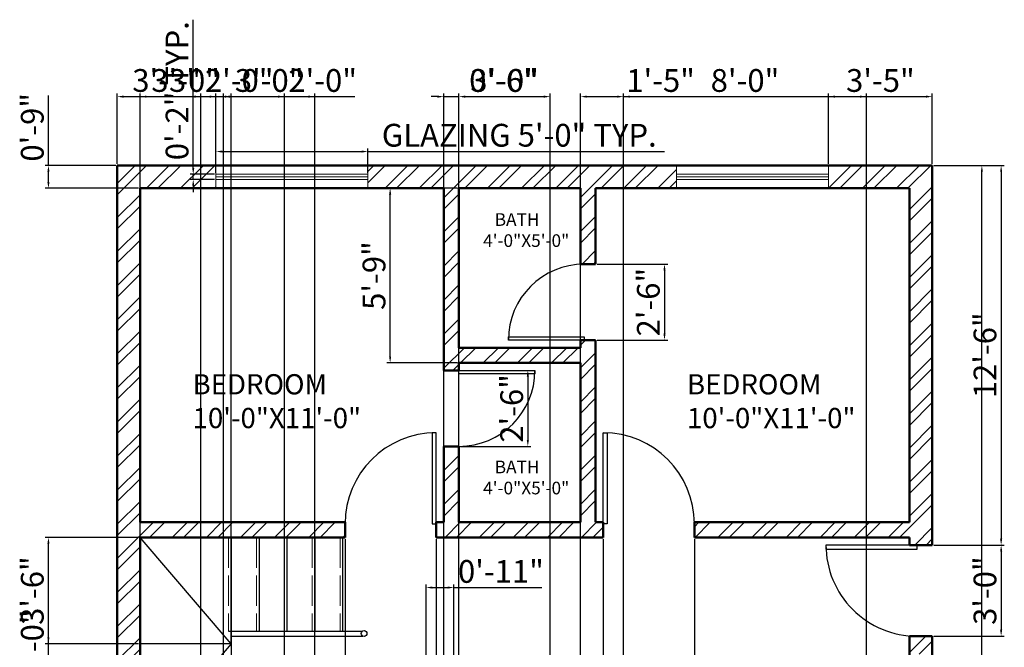
# Model space of a CAD drawing. Units: inches. Extents: x 234 to 630, y 1038 to 1631.
# Tile 2 of 2: x 234 to 623, y 1383 to 1631. Entities that reach past the tile are written whole.
import ezdxf

# ---------------------------------------------------------------- set-up
doc = ezdxf.new("R2010")
doc.units = ezdxf.units.IN
doc.linetypes.add('ACAD_ISO02W100', pattern=[15, 12, -3])
for name, color, linetype, lineweight in [('A-ANNO-DIMS', 2, 'Continuous', 18), ('A-AREA-IDEN', 7, 'Continuous', 25), ('A-DOOR', 4, 'Continuous', 25), ('A-FLOR-STRS', 7, 'Continuous', 25), ('A-FLOR-STRS-HIDN', 8, 'ACAD_ISO02W100', 13), ('A-GLAZ', 244, 'Continuous', 18), ('A-WALL', 7, 'Continuous', 50), ('A-WALL-PATT', 252, 'Continuous', 13)]:
    doc.layers.add(name, color=color, linetype=linetype, lineweight=lineweight)
doc.styles.get("Standard").update_dxf_attribs({"font": 'arial.ttf'})
doc.dimstyles.new('ISO-25', dxfattribs={"dimtxt": 9, "dimasz": 2.5, "dimexe": 1.25, "dimexo": 0.625, "dimtad": 1, "dimlunit": 3, "dimtxsty": 'Standard', "dimcen": 2.5, "dimadec": 0, "dimazin": 0, "dimtfac": 1, "dimtmove": 0, "dimatfit": 3, "dimfxl": 1, "dimarcsym": 0})

# ---------------------------------------------------------------- blocks, each defined once
blk = doc.blocks.new('*U2')
for p, q in [((0, 0), (0, -6)), ((40, 0), (40, -6))]:
    blk.add_line(p, q)
blk.add_lwpolyline([(0, 0), (0, 40), (1.75, 40), (1.75, 0)], close=True)
blk.add_arc((0, 0), 40, 0, 90)
blk = doc.blocks.new('*U4')
for p, q in [((0, 0), (0, -6)), ((-40, 0), (-40, -6))]:
    blk.add_line(p, q)
blk.add_lwpolyline([(0, 0), (0, 40), (-1.75, 40), (-1.75, 0)], close=True)
blk.add_arc((0, 0), 40, 90, 180)
blk = doc.blocks.new('*U5')
for p, q in [((-40, 0), (-40, 6)), ((0, 0), (0, 6))]:
    blk.add_line(p, q)
blk.add_lwpolyline([(0, 0), (0, -40), (-1.75, -40), (-1.75, 0)], close=True)
blk.add_arc((0, 0), 40, 180, 270)
blk = doc.blocks.new('*U3')
for p, q in [((0, 0), (0, 6)), ((40, 0), (40, 6))]:
    blk.add_line(p, q)
blk.add_lwpolyline([(0, 0), (0, -40), (1.75, -40), (1.75, 0)], close=True)
blk.add_arc((0, 0), 40, 270, 0)
blk = doc.blocks.new('*D9')
at = {"layer": 'A-ANNO-DIMS', "color": 0, "lineweight": -2, "transparency": 16777216}
for p, q in [((595.56, 1573.18), (615.76, 1573.18)), ((614.51, 1074.68), (614.51, 1570.68)), ((595.56, 1072.18), (615.76, 1072.18))]:
    blk.add_line(p, q, dxfattribs=at)
at = {"layer": 'A-ANNO-DIMS', "color": 0, "transparency": 16777216}
for points in [[(614.09, 1570.68), (614.92, 1570.68), (614.51, 1573.18)], [(614.09, 1074.68), (614.92, 1074.68), (614.51, 1072.18)]]:
    blk.add_solid(points, dxfattribs=at)
at = {"layer": 'Defpoints', "color": 0, "transparency": 16777216}
for p in [(594.93, 1573.18), (614.51, 1573.18), (594.93, 1072.18)]:
    blk.add_point(p, dxfattribs=at)
at = {"layer": 'A-ANNO-DIMS', "color": 0, "transparency": 16777216, "insert": (609.29, 1322.68), "char_height": 9, "attachment_point": 5, "rotation": 90}
blk.add_mtext('41\'-9"', dxfattribs=at)
blk = doc.blocks.new('WIN-GLAZING-60IN')
for p, q in [((0, 2), (60, 2)), ((0, 1), (60, 1)), ((0, 0), (60, 0))]:
    blk.add_line(p, q)
blk = doc.blocks.new('*D11')
at = {"layer": 'A-ANNO-DIMS', "color": 0, "lineweight": -2, "transparency": 16777216}
for p, q in [((311.93, 1570.3), (311.93, 1579.93)), ((371.93, 1570.3), (371.93, 1579.93)), ((314.43, 1578.68), (369.43, 1578.68)), ((371.93, 1578.68), (489.08, 1578.68))]:
    blk.add_line(p, q, dxfattribs=at)
at = {"layer": 'A-ANNO-DIMS', "color": 0, "transparency": 16777216}
for points in [[(314.43, 1579.1), (314.43, 1578.26), (311.93, 1578.68)], [(369.43, 1579.1), (369.43, 1578.26), (371.93, 1578.68)]]:
    blk.add_solid(points, dxfattribs=at)
at = {"layer": 'Defpoints', "color": 0, "transparency": 16777216}
for p in [(371.93, 1578.68), (311.93, 1569.68), (371.93, 1569.68)]:
    blk.add_point(p, dxfattribs=at)
at = {"layer": 'A-ANNO-DIMS', "color": 0, "transparency": 16777216, "insert": (431.75, 1583.96), "char_height": 9, "attachment_point": 5}
blk.add_mtext('GLAZING 5\'-0" TYP.', dxfattribs=at)
blk = doc.blocks.new('*D12')
at = {"layer": 'A-ANNO-DIMS', "color": 0, "lineweight": -2, "transparency": 16777216}
for p, q in [((302.93, 1572.18), (302.93, 1630.79)), ((311.31, 1569.68), (301.68, 1569.68)), ((302.93, 1567.68), (302.93, 1569.68)), ((311.31, 1567.68), (301.68, 1567.68)), ((302.93, 1565.18), (302.93, 1562.68))]:
    blk.add_line(p, q, dxfattribs=at)
at = {"layer": 'A-ANNO-DIMS', "color": 0, "transparency": 16777216}
for points in [[(302.51, 1572.18), (303.35, 1572.18), (302.93, 1569.68)], [(302.51, 1565.18), (303.35, 1565.18), (302.93, 1567.68)]]:
    blk.add_solid(points, dxfattribs=at)
at = {"layer": 'Defpoints', "color": 0, "transparency": 16777216}
for p in [(302.93, 1569.68), (311.93, 1569.68), (311.93, 1567.68)]:
    blk.add_point(p, dxfattribs=at)
at = {"layer": 'A-ANNO-DIMS', "color": 0, "transparency": 16777216, "insert": (297.71, 1602.73), "char_height": 9, "attachment_point": 5, "rotation": 90}
blk.add_mtext('0\'-2" TYP.', dxfattribs=at)
blk = doc.blocks.new('*D13')
at = {"layer": 'A-ANNO-DIMS', "color": 0, "lineweight": -2, "transparency": 16777216}
for p, q in [((272.93, 1573.8), (272.93, 1601.63)), ((275.43, 1600.38), (309.43, 1600.38)), ((311.93, 1573.8), (311.93, 1601.63))]:
    blk.add_line(p, q, dxfattribs=at)
at = {"layer": 'A-ANNO-DIMS', "color": 0, "transparency": 16777216}
for points in [[(275.43, 1600.8), (275.43, 1599.96), (272.93, 1600.38)], [(309.43, 1600.8), (309.43, 1599.96), (311.93, 1600.38)]]:
    blk.add_solid(points, dxfattribs=at)
at = {"layer": 'Defpoints', "color": 0, "transparency": 16777216}
for p in [(311.93, 1600.38), (272.93, 1573.18), (311.93, 1573.18)]:
    blk.add_point(p, dxfattribs=at)
at = {"layer": 'A-ANNO-DIMS', "color": 0, "transparency": 16777216, "insert": (292.43, 1605.6), "char_height": 9, "attachment_point": 5}
blk.add_mtext('3\'-3"', dxfattribs=at)
blk = doc.blocks.new('*D14')
at = {"layer": 'A-ANNO-DIMS', "color": 0, "lineweight": -2, "transparency": 16777216}
for p, q in [((553.93, 1573.8), (553.93, 1601.63)), ((556.43, 1600.38), (592.43, 1600.38)), ((594.93, 1573.8), (594.93, 1601.63))]:
    blk.add_line(p, q, dxfattribs=at)
at = {"layer": 'A-ANNO-DIMS', "color": 0, "transparency": 16777216}
for points in [[(556.43, 1600.8), (556.43, 1599.96), (553.93, 1600.38)], [(592.43, 1600.8), (592.43, 1599.96), (594.93, 1600.38)]]:
    blk.add_solid(points, dxfattribs=at)
at = {"layer": 'Defpoints', "color": 0, "transparency": 16777216}
for p in [(594.93, 1600.38), (553.93, 1573.18), (594.93, 1573.18)]:
    blk.add_point(p, dxfattribs=at)
at = {"layer": 'A-ANNO-DIMS', "color": 0, "transparency": 16777216, "insert": (574.43, 1605.6), "char_height": 9, "attachment_point": 5}
blk.add_mtext('3\'-5"', dxfattribs=at)
blk = doc.blocks.new('*D15')
at = {"layer": 'A-ANNO-DIMS', "color": 0, "lineweight": -2, "transparency": 16777216}
for p, q in [((245.73, 1573.18), (245.73, 1600.85)), ((272.31, 1573.18), (244.48, 1573.18)), ((245.73, 1566.68), (245.73, 1570.68)), ((281.31, 1564.18), (244.48, 1564.18))]:
    blk.add_line(p, q, dxfattribs=at)
at = {"layer": 'A-ANNO-DIMS', "color": 0, "transparency": 16777216}
for points in [[(245.31, 1570.68), (246.15, 1570.68), (245.73, 1573.18)], [(245.31, 1566.68), (246.15, 1566.68), (245.73, 1564.18)]]:
    blk.add_solid(points, dxfattribs=at)
at = {"layer": 'Defpoints', "color": 0, "transparency": 16777216}
for p in [(245.73, 1573.18), (272.93, 1573.18), (281.93, 1564.18)]:
    blk.add_point(p, dxfattribs=at)
at = {"layer": 'A-ANNO-DIMS', "color": 0, "transparency": 16777216, "insert": (240.51, 1588.27), "char_height": 9, "attachment_point": 5, "rotation": 90}
blk.add_mtext('0\'-9"', dxfattribs=at)
blk = doc.blocks.new('*D16')
at = {"layer": 'A-ANNO-DIMS', "color": 0, "lineweight": -2, "transparency": 16777216}
for p, q in [((281.31, 1426.18), (244.48, 1426.18)), ((245.73, 1344.68), (245.73, 1423.68)), ((281.31, 1342.18), (244.48, 1342.18))]:
    blk.add_line(p, q, dxfattribs=at)
at = {"layer": 'A-ANNO-DIMS', "color": 0, "transparency": 16777216}
for points in [[(245.31, 1423.68), (246.15, 1423.68), (245.73, 1426.18)], [(245.31, 1344.68), (246.15, 1344.68), (245.73, 1342.18)]]:
    blk.add_solid(points, dxfattribs=at)
at = {"layer": 'Defpoints', "color": 0, "transparency": 16777216}
for p in [(245.73, 1426.18), (281.93, 1426.18), (281.93, 1342.18)]:
    blk.add_point(p, dxfattribs=at)
at = {"layer": 'A-ANNO-DIMS', "color": 0, "transparency": 16777216, "insert": (240.51, 1384.18), "char_height": 9, "attachment_point": 5, "rotation": 90}
blk.add_mtext('7\'-0"', dxfattribs=at)
blk = doc.blocks.new('*D18')
at = {"layer": 'A-ANNO-DIMS', "color": 0, "lineweight": -2, "transparency": 16777216}
for p, q in [((595.56, 1573.18), (623.38, 1573.18)), ((622.13, 1570.68), (622.13, 1425.68)), ((595.56, 1423.18), (623.38, 1423.18))]:
    blk.add_line(p, q, dxfattribs=at)
at = {"layer": 'A-ANNO-DIMS', "color": 0, "transparency": 16777216}
for points in [[(621.71, 1570.68), (622.55, 1570.68), (622.13, 1573.18)], [(621.71, 1425.68), (622.55, 1425.68), (622.13, 1423.18)]]:
    blk.add_solid(points, dxfattribs=at)
at = {"layer": 'Defpoints', "color": 0, "transparency": 16777216}
for p in [(594.93, 1573.18), (594.93, 1423.18), (622.13, 1423.18)]:
    blk.add_point(p, dxfattribs=at)
at = {"layer": 'A-ANNO-DIMS', "color": 0, "transparency": 16777216, "insert": (616.91, 1498.18), "char_height": 9, "attachment_point": 5, "rotation": 90}
blk.add_mtext('12\'-6"', dxfattribs=at)
blk = doc.blocks.new('*D19')
at = {"layer": 'A-ANNO-DIMS', "color": 0, "lineweight": -2, "transparency": 16777216}
for p, q in [((595.56, 1423.18), (623.38, 1423.18)), ((622.13, 1420.68), (622.13, 1389.68)), ((595.56, 1387.18), (623.38, 1387.18))]:
    blk.add_line(p, q, dxfattribs=at)
at = {"layer": 'A-ANNO-DIMS', "color": 0, "transparency": 16777216}
for points in [[(621.71, 1420.68), (622.55, 1420.68), (622.13, 1423.18)], [(621.71, 1389.68), (622.55, 1389.68), (622.13, 1387.18)]]:
    blk.add_solid(points, dxfattribs=at)
at = {"layer": 'Defpoints', "color": 0, "transparency": 16777216}
for p in [(594.93, 1423.18), (594.93, 1387.18), (622.13, 1387.18)]:
    blk.add_point(p, dxfattribs=at)
at = {"layer": 'A-ANNO-DIMS', "color": 0, "transparency": 16777216, "insert": (616.91, 1405.18), "char_height": 9, "attachment_point": 5, "rotation": 90}
blk.add_mtext('3\'-0"', dxfattribs=at)
blk = doc.blocks.new('*D22')
at = {"layer": 'A-ANNO-DIMS', "color": 0, "lineweight": -2, "transparency": 16777216}
for p, q in [((281.93, 1078.8), (281.93, 1601.63)), ((284.43, 1600.38), (303.43, 1600.38)), ((305.93, 1102.8), (305.93, 1601.63)), ((305.93, 1600.38), (333.76, 1600.38))]:
    blk.add_line(p, q, dxfattribs=at)
at = {"layer": 'A-ANNO-DIMS', "color": 0, "transparency": 16777216}
for points in [[(284.43, 1600.8), (284.43, 1599.96), (281.93, 1600.38)], [(303.43, 1600.8), (303.43, 1599.96), (305.93, 1600.38)]]:
    blk.add_solid(points, dxfattribs=at)
at = {"layer": 'Defpoints', "color": 0, "transparency": 16777216}
for p in [(305.93, 1600.38), (305.93, 1102.18), (281.93, 1078.18)]:
    blk.add_point(p, dxfattribs=at)
at = {"layer": 'A-ANNO-DIMS', "color": 0, "transparency": 16777216, "insert": (321.09, 1605.6), "char_height": 9, "attachment_point": 5}
blk.add_mtext('2\'-0"', dxfattribs=at)
blk = doc.blocks.new('*D24')
at = {"layer": 'A-ANNO-DIMS', "color": 0, "lineweight": -2, "transparency": 16777216}
for p, q in [((472.93, 1078.8), (472.93, 1601.63)), ((475.43, 1600.38), (566.43, 1600.38)), ((568.93, 1078.8), (568.93, 1601.63))]:
    blk.add_line(p, q, dxfattribs=at)
at = {"layer": 'A-ANNO-DIMS', "color": 0, "transparency": 16777216}
for points in [[(475.43, 1600.8), (475.43, 1599.96), (472.93, 1600.38)], [(566.43, 1600.8), (566.43, 1599.96), (568.93, 1600.38)]]:
    blk.add_solid(points, dxfattribs=at)
at = {"layer": 'Defpoints', "color": 0, "transparency": 16777216}
for p in [(568.93, 1600.38), (472.93, 1078.18), (568.93, 1078.18)]:
    blk.add_point(p, dxfattribs=at)
at = {"layer": 'A-ANNO-DIMS', "color": 0, "transparency": 16777216, "insert": (520.93, 1605.6), "char_height": 9, "attachment_point": 5}
blk.add_mtext('8\'-0"', dxfattribs=at)
blk = doc.blocks.new('*D25')
at = {"layer": 'A-ANNO-DIMS', "color": 0, "lineweight": -2, "transparency": 16777216}
for p, q in [((455.93, 1078.8), (455.93, 1601.63)), ((458.43, 1600.38), (470.43, 1600.38)), ((472.93, 1078.8), (472.93, 1601.63)), ((472.93, 1600.38), (499.76, 1600.38))]:
    blk.add_line(p, q, dxfattribs=at)
at = {"layer": 'A-ANNO-DIMS', "color": 0, "transparency": 16777216}
for points in [[(458.43, 1600.8), (458.43, 1599.96), (455.93, 1600.38)], [(470.43, 1600.8), (470.43, 1599.96), (472.93, 1600.38)]]:
    blk.add_solid(points, dxfattribs=at)
at = {"layer": 'Defpoints', "color": 0, "transparency": 16777216}
for p in [(472.93, 1600.38), (455.93, 1078.18), (472.93, 1078.18)]:
    blk.add_point(p, dxfattribs=at)
at = {"layer": 'A-ANNO-DIMS', "color": 0, "transparency": 16777216, "insert": (487.59, 1605.6), "char_height": 9, "attachment_point": 5}
blk.add_mtext('1\'-5"', dxfattribs=at)
blk = doc.blocks.new('*D28')
at = {"layer": 'A-ANNO-DIMS', "color": 0, "lineweight": -2, "transparency": 16777216}
for p, q in [((407.93, 1207.8), (407.93, 1601.63)), ((410.43, 1600.38), (441.43, 1600.38)), ((443.93, 1207.8), (443.93, 1601.63))]:
    blk.add_line(p, q, dxfattribs=at)
at = {"layer": 'A-ANNO-DIMS', "color": 0, "transparency": 16777216}
for points in [[(410.43, 1600.8), (410.43, 1599.96), (407.93, 1600.38)], [(441.43, 1600.8), (441.43, 1599.96), (443.93, 1600.38)]]:
    blk.add_solid(points, dxfattribs=at)
at = {"layer": 'Defpoints', "color": 0, "transparency": 16777216}
for p in [(443.93, 1600.38), (407.93, 1207.18), (443.93, 1207.18)]:
    blk.add_point(p, dxfattribs=at)
at = {"layer": 'A-ANNO-DIMS', "color": 0, "transparency": 16777216, "insert": (425.93, 1605.6), "char_height": 9, "attachment_point": 5}
blk.add_mtext('3\'-0"', dxfattribs=at)
blk = doc.blocks.new('*D29')
at = {"layer": 'A-ANNO-DIMS', "color": 0, "lineweight": -2, "transparency": 16777216}
for p, q in [((314.93, 1111.8), (314.93, 1601.63)), ((317.43, 1600.38), (348.43, 1600.38)), ((350.93, 1111.8), (350.93, 1601.63))]:
    blk.add_line(p, q, dxfattribs=at)
at = {"layer": 'A-ANNO-DIMS', "color": 0, "transparency": 16777216}
for points in [[(317.43, 1600.8), (317.43, 1599.96), (314.93, 1600.38)], [(348.43, 1600.8), (348.43, 1599.96), (350.93, 1600.38)]]:
    blk.add_solid(points, dxfattribs=at)
at = {"layer": 'Defpoints', "color": 0, "transparency": 16777216}
for p in [(350.93, 1600.38), (314.93, 1111.18), (350.93, 1111.18)]:
    blk.add_point(p, dxfattribs=at)
at = {"layer": 'A-ANNO-DIMS', "color": 0, "transparency": 16777216, "insert": (332.93, 1605.6), "char_height": 9, "attachment_point": 5}
blk.add_mtext('3\'-0"', dxfattribs=at)
blk = doc.blocks.new('*D30')
at = {"layer": 'A-ANNO-DIMS', "color": 0, "lineweight": -2, "transparency": 16777216}
for p, q in [((314.93, 1168.81), (314.93, 1601.63)), ((317.43, 1600.38), (336.43, 1600.38)), ((338.93, 1168.81), (338.93, 1601.63)), ((338.93, 1600.38), (366.76, 1600.38))]:
    blk.add_line(p, q, dxfattribs=at)
at = {"layer": 'A-ANNO-DIMS', "color": 0, "transparency": 16777216}
for points in [[(317.43, 1600.8), (317.43, 1599.96), (314.93, 1600.38)], [(336.43, 1600.8), (336.43, 1599.96), (338.93, 1600.38)]]:
    blk.add_solid(points, dxfattribs=at)
at = {"layer": 'Defpoints', "color": 0, "transparency": 16777216}
for p in [(338.93, 1600.38), (314.93, 1168.18), (338.93, 1168.18)]:
    blk.add_point(p, dxfattribs=at)
at = {"layer": 'A-ANNO-DIMS', "color": 0, "transparency": 16777216, "insert": (354.09, 1605.6), "char_height": 9, "attachment_point": 5}
blk.add_mtext('2\'-0"', dxfattribs=at)
blk = doc.blocks.new('*D32')
at = {"layer": 'A-ANNO-DIMS', "color": 0, "lineweight": -2, "transparency": 16777216}
for p, q in [((399.43, 1600.38), (396.93, 1600.38)), ((401.93, 1297.8), (401.93, 1601.63)), ((401.93, 1600.38), (407.93, 1600.38)), ((407.93, 1297.8), (407.93, 1601.63)), ((410.43, 1600.38), (438.1, 1600.38))]:
    blk.add_line(p, q, dxfattribs=at)
at = {"layer": 'A-ANNO-DIMS', "color": 0, "transparency": 16777216}
for points in [[(399.43, 1600.8), (399.43, 1599.96), (401.93, 1600.38)], [(410.43, 1600.8), (410.43, 1599.96), (407.93, 1600.38)]]:
    blk.add_solid(points, dxfattribs=at)
at = {"layer": 'Defpoints', "color": 0, "transparency": 16777216}
for p in [(407.93, 1600.38), (401.93, 1297.18), (407.93, 1297.18)]:
    blk.add_point(p, dxfattribs=at)
at = {"layer": 'A-ANNO-DIMS', "color": 0, "transparency": 16777216, "insert": (425.52, 1605.6), "char_height": 9, "attachment_point": 5}
blk.add_mtext('0\'-6"', dxfattribs=at)
blk = doc.blocks.new('*D33')
at = {"layer": 'A-ANNO-DIMS', "color": 0, "lineweight": -2, "transparency": 16777216}
for p, q in [((281.93, 1384.8), (281.93, 1601.63)), ((284.43, 1600.38), (315.43, 1600.38)), ((317.93, 1384.8), (317.93, 1601.63))]:
    blk.add_line(p, q, dxfattribs=at)
at = {"layer": 'A-ANNO-DIMS', "color": 0, "transparency": 16777216}
for points in [[(284.43, 1600.8), (284.43, 1599.96), (281.93, 1600.38)], [(315.43, 1600.8), (315.43, 1599.96), (317.93, 1600.38)]]:
    blk.add_solid(points, dxfattribs=at)
at = {"layer": 'Defpoints', "color": 0, "transparency": 16777216}
for p in [(317.93, 1600.38), (281.93, 1384.18), (317.93, 1384.18)]:
    blk.add_point(p, dxfattribs=at)
at = {"layer": 'A-ANNO-DIMS', "color": 0, "transparency": 16777216, "insert": (299.93, 1605.6), "char_height": 9, "attachment_point": 5}
blk.add_mtext('3\'-0"', dxfattribs=at)
blk = doc.blocks.new('*D34')
at = {"layer": 'A-ANNO-DIMS', "color": 0, "lineweight": -2, "transparency": 16777216}
for p, q in [((362.93, 1425.55), (362.93, 1043.73)), ((398.93, 1425.55), (398.93, 1043.73)), ((365.43, 1044.98), (396.43, 1044.98))]:
    blk.add_line(p, q, dxfattribs=at)
at = {"layer": 'A-ANNO-DIMS', "color": 0, "transparency": 16777216}
for points in [[(365.43, 1045.4), (365.43, 1044.56), (362.93, 1044.98)], [(396.43, 1045.4), (396.43, 1044.56), (398.93, 1044.98)]]:
    blk.add_solid(points, dxfattribs=at)
at = {"layer": 'Defpoints', "color": 0, "transparency": 16777216}
for p in [(362.93, 1426.18), (398.93, 1426.18), (398.93, 1044.98)]:
    blk.add_point(p, dxfattribs=at)
at = {"layer": 'A-ANNO-DIMS', "color": 0, "transparency": 16777216, "insert": (380.93, 1050.2), "char_height": 9, "attachment_point": 5}
blk.add_mtext('3\'-0"', dxfattribs=at)
blk = doc.blocks.new('*D35')
at = {"layer": 'A-ANNO-DIMS', "color": 0, "lineweight": -2, "transparency": 16777216}
for p, q in [((464.93, 1425.55), (464.93, 1043.73)), ((500.93, 1425.55), (500.93, 1043.73)), ((467.43, 1044.98), (498.43, 1044.98))]:
    blk.add_line(p, q, dxfattribs=at)
at = {"layer": 'A-ANNO-DIMS', "color": 0, "transparency": 16777216}
for points in [[(467.43, 1045.4), (467.43, 1044.56), (464.93, 1044.98)], [(498.43, 1045.4), (498.43, 1044.56), (500.93, 1044.98)]]:
    blk.add_solid(points, dxfattribs=at)
at = {"layer": 'Defpoints', "color": 0, "transparency": 16777216}
for p in [(464.93, 1426.18), (500.93, 1426.18), (500.93, 1044.98)]:
    blk.add_point(p, dxfattribs=at)
at = {"layer": 'A-ANNO-DIMS', "color": 0, "transparency": 16777216, "insert": (482.93, 1050.2), "char_height": 9, "attachment_point": 5}
blk.add_mtext('3\'-0"', dxfattribs=at)
blk = doc.blocks.new('*D36')
at = {"layer": 'A-ANNO-DIMS', "color": 0, "lineweight": -2, "transparency": 16777216}
for p, q in [((408.56, 1492.18), (436.38, 1492.18)), ((435.13, 1489.68), (435.13, 1464.68)), ((408.56, 1462.18), (436.38, 1462.18))]:
    blk.add_line(p, q, dxfattribs=at)
at = {"layer": 'A-ANNO-DIMS', "color": 0, "transparency": 16777216}
for points in [[(434.71, 1489.68), (435.55, 1489.68), (435.13, 1492.18)], [(434.71, 1464.68), (435.55, 1464.68), (435.13, 1462.18)]]:
    blk.add_solid(points, dxfattribs=at)
at = {"layer": 'Defpoints', "color": 0, "transparency": 16777216}
for p in [(407.93, 1492.18), (407.93, 1462.18), (435.13, 1462.18)]:
    blk.add_point(p, dxfattribs=at)
at = {"layer": 'A-ANNO-DIMS', "color": 0, "transparency": 16777216, "insert": (429.91, 1477.18), "char_height": 9, "attachment_point": 5, "rotation": 90}
blk.add_mtext('2\'-6"', dxfattribs=at)
blk = doc.blocks.new('*D37')
at = {"layer": 'A-ANNO-DIMS', "color": 0, "lineweight": -2, "transparency": 16777216}
for p, q in [((462.56, 1534.18), (490.38, 1534.18)), ((489.13, 1531.68), (489.13, 1506.68)), ((462.56, 1504.18), (490.38, 1504.18))]:
    blk.add_line(p, q, dxfattribs=at)
at = {"layer": 'A-ANNO-DIMS', "color": 0, "transparency": 16777216}
for points in [[(488.71, 1531.68), (489.55, 1531.68), (489.13, 1534.18)], [(488.71, 1506.68), (489.55, 1506.68), (489.13, 1504.18)]]:
    blk.add_solid(points, dxfattribs=at)
at = {"layer": 'Defpoints', "color": 0, "transparency": 16777216}
for p in [(461.93, 1534.18), (461.93, 1504.18), (489.13, 1504.18)]:
    blk.add_point(p, dxfattribs=at)
at = {"layer": 'A-ANNO-DIMS', "color": 0, "transparency": 16777216, "insert": (483.91, 1519.18), "char_height": 9, "attachment_point": 5, "rotation": 90}
blk.add_mtext('2\'-6"', dxfattribs=at)
blk = doc.blocks.new('*D40')
at = {"layer": 'A-ANNO-DIMS', "color": 0, "lineweight": -2, "transparency": 16777216}
for p, q in [((394.93, 1379.8), (394.93, 1407.63)), ((397.43, 1406.38), (403.43, 1406.38)), ((405.93, 1379.8), (405.93, 1407.63)), ((405.93, 1406.38), (440.6, 1406.38))]:
    blk.add_line(p, q, dxfattribs=at)
at = {"layer": 'A-ANNO-DIMS', "color": 0, "transparency": 16777216}
for points in [[(397.43, 1406.8), (397.43, 1405.96), (394.93, 1406.38)], [(403.43, 1406.8), (403.43, 1405.96), (405.93, 1406.38)]]:
    blk.add_solid(points, dxfattribs=at)
at = {"layer": 'Defpoints', "color": 0, "transparency": 16777216}
for p in [(405.93, 1406.38), (394.93, 1379.18), (405.93, 1379.18)]:
    blk.add_point(p, dxfattribs=at)
at = {"layer": 'A-ANNO-DIMS', "color": 0, "transparency": 16777216, "insert": (424.51, 1411.6), "char_height": 9, "attachment_point": 5}
blk.add_mtext('0\'-11"', dxfattribs=at)
blk = doc.blocks.new('*D41')
at = {"layer": 'A-ANNO-DIMS', "color": 0, "lineweight": -2, "transparency": 16777216}
for p, q in [((281.31, 1426.18), (244.48, 1426.18)), ((245.73, 1386.68), (245.73, 1423.68)), ((281.31, 1384.18), (244.48, 1384.18))]:
    blk.add_line(p, q, dxfattribs=at)
at = {"layer": 'A-ANNO-DIMS', "color": 0, "transparency": 16777216}
for points in [[(245.31, 1423.68), (246.15, 1423.68), (245.73, 1426.18)], [(245.31, 1386.68), (246.15, 1386.68), (245.73, 1384.18)]]:
    blk.add_solid(points, dxfattribs=at)
at = {"layer": 'Defpoints', "color": 0, "transparency": 16777216}
for p in [(245.73, 1426.18), (281.93, 1426.18), (281.93, 1384.18)]:
    blk.add_point(p, dxfattribs=at)
at = {"layer": 'A-ANNO-DIMS', "color": 0, "transparency": 16777216, "insert": (240.51, 1405.18), "char_height": 9, "attachment_point": 5, "rotation": 90}
blk.add_mtext('3\'-6"', dxfattribs=at)
blk = doc.blocks.new('*D43')
at = {"layer": 'A-ANNO-DIMS', "color": 0, "lineweight": -2, "transparency": 16777216}
for p, q in [((407.31, 1564.18), (379.48, 1564.18)), ((380.73, 1497.68), (380.73, 1561.68)), ((407.31, 1495.18), (379.48, 1495.18))]:
    blk.add_line(p, q, dxfattribs=at)
at = {"layer": 'A-ANNO-DIMS', "color": 0, "transparency": 16777216}
for points in [[(380.31, 1561.68), (381.15, 1561.68), (380.73, 1564.18)], [(380.31, 1497.68), (381.15, 1497.68), (380.73, 1495.18)]]:
    blk.add_solid(points, dxfattribs=at)
at = {"layer": 'Defpoints', "color": 0, "transparency": 16777216}
for p in [(380.73, 1564.18), (407.93, 1564.18), (407.93, 1495.18)]:
    blk.add_point(p, dxfattribs=at)
at = {"layer": 'A-ANNO-DIMS', "color": 0, "transparency": 16777216, "insert": (375.51, 1529.68), "char_height": 9, "attachment_point": 5, "rotation": 90}
blk.add_mtext('5\'-9"', dxfattribs=at)

msp = doc.modelspace()

# ---------------------------------------------------------------- hatches: boundary and pattern name
at = {"layer": 'A-WALL-PATT'}
h = msp.add_hatch(dxfattribs=at)
h.set_pattern_fill('ANSI32', color=256)
h.paths.add_polyline_path([(407.931, 1216.178), (407.931, 1297.178), (401.931, 1297.178), (401.931, 1213.178), (281.931, 1213.178), (281.931, 1336.178), (284.931, 1336.178), (284.931, 1342.178), (281.931, 1342.178), (281.931, 1426.178), (362.931, 1426.178), (362.931, 1432.178), (281.931, 1432.178), (281.931, 1564.178), (311.931, 1564.178), (311.931, 1573.178), (272.931, 1573.178), (272.931, 1072.178), (455.931, 1072.178), (455.931, 1102.178), (455.931, 1207.178), (458.931, 1207.178), (458.931, 1216.178), (443.931, 1216.178), (443.931, 1207.178), (446.931, 1207.178), (446.931, 1111.178), (410.931, 1111.178), (410.931, 1102.178), (452.931, 1102.178), (452.931, 1078.178), (281.931, 1078.178), (281.931, 1207.178), (305.931, 1207.178), (305.931, 1204.178), (314.931, 1204.178), (314.931, 1207.178), (407.931, 1207.178)])
h.paths.add_polyline_path([(314.931, 1174.178), (305.931, 1174.178), (305.931, 1102.178), (350.931, 1102.178), (350.931, 1111.178), (314.931, 1111.178)], flags=17)
h.paths.add_polyline_path([(493.931, 1573.178), (371.931, 1573.178), (371.931, 1564.178), (401.931, 1564.178), (401.931, 1492.178), (407.931, 1492.178), (407.931, 1495.178), (455.931, 1495.178), (455.931, 1432.178), (407.931, 1432.178), (407.931, 1462.178), (401.931, 1462.178), (401.931, 1432.178), (398.931, 1432.178), (398.931, 1426.178), (464.931, 1426.178), (464.931, 1432.178), (461.931, 1432.178), (461.931, 1504.178), (455.931, 1504.178), (455.931, 1501.178), (407.931, 1501.178), (407.931, 1564.178), (455.931, 1564.178), (455.931, 1534.178), (461.931, 1534.178), (461.931, 1564.178), (493.931, 1564.178)])
h.paths.add_polyline_path([(594.931, 1573.178), (553.931, 1573.178), (553.931, 1564.178), (585.931, 1564.178), (585.931, 1432.178), (500.931, 1432.178), (500.931, 1426.178), (585.931, 1426.178), (585.931, 1423.178), (594.931, 1423.178)])
h.paths.add_polyline_path([(594.931, 1320.043), (585.931, 1320.043), (585.931, 1303.302), (594.931, 1303.302)])
h.paths.add_polyline_path([(594.931, 1387.178), (585.931, 1387.178), (585.931, 1380.043), (594.931, 1380.043)])
h.paths.add_polyline_path([(594.931, 1243.302), (585.931, 1243.302), (585.931, 1216.178), (580.931, 1216.178), (580.931, 1207.178), (594.931, 1207.178)])
h.paths.add_polyline_path([(520.931, 1216.178), (506.931, 1216.178), (506.931, 1207.178), (520.931, 1207.178)])

# ---------------------------------------------------------------- linework, layer by layer
at = {"layer": 'A-FLOR-STRS'}
for p, q in [((317.931, 1384.178), (281.931, 1426.178)), ((317.931, 1426.178), (317.931, 1342.178)), ((328.931, 1426.178), (328.931, 1389.178)), ((339.931, 1426.178), (339.931, 1389.178)), ((350.931, 1426.178), (350.931, 1389.178)), ((361.931, 1426.178), (361.931, 1389.178)), ((316.931, 1389.178), (369.809, 1389.178)), ((317.931, 1387.178), (370.007, 1387.178)), ((317.931, 1384.178), (281.931, 1384.178)), ((317.931, 1384.178), (281.931, 1342.178))]:
    msp.add_line(p, q, dxfattribs=at)
msp.add_circle((370.43, 1388.23), 1.134, dxfattribs=at)
at = {"layer": 'A-FLOR-STRS-HIDN'}
for p, q in [((316.931, 1426.178), (316.931, 1389.178)), ((327.931, 1426.178), (327.931, 1389.178)), ((338.931, 1426.178), (338.931, 1389.178)), ((349.931, 1426.178), (349.931, 1389.178)), ((360.931, 1426.178), (360.931, 1389.178))]:
    msp.add_line(p, q, dxfattribs=at)
at = {"layer": 'A-GLAZ'}
for points in [[(311.931, 1573.178), (371.931, 1573.178), (371.931, 1564.178), (311.931, 1564.178)], [(493.931, 1573.178), (553.931, 1573.178), (553.931, 1564.178), (493.931, 1564.178)]]:
    msp.add_lwpolyline(points, close=True, dxfattribs=at)
at = {"layer": 'A-WALL'}
for p, q in [((272.931, 1573.178), (272.931, 1072.178)), ((272.931, 1573.178), (594.931, 1573.178)), ((594.931, 1573.178), (594.931, 1423.178)), ((281.931, 1564.178), (281.931, 1432.178)), ((281.931, 1564.178), (401.931, 1564.178)), ((401.931, 1564.178), (401.931, 1492.178)), ((407.931, 1564.178), (407.931, 1501.178)), ((407.931, 1564.178), (455.931, 1564.178)), ((455.931, 1564.178), (455.931, 1534.178)), ((461.931, 1564.178), (461.931, 1534.178)), ((461.931, 1564.178), (585.931, 1564.178)), ((585.931, 1564.178), (585.931, 1432.178)), ((455.931, 1534.178), (461.931, 1534.178)), ((455.931, 1504.178), (461.931, 1504.178)), ((455.931, 1504.178), (455.931, 1501.178)), ((461.931, 1504.178), (461.931, 1432.178)), ((407.931, 1501.178), (455.931, 1501.178)), ((407.931, 1495.178), (455.931, 1495.178)), ((407.931, 1495.178), (407.931, 1492.178)), ((455.931, 1495.178), (455.931, 1432.178)), ((407.931, 1492.178), (401.931, 1492.178)), ((407.931, 1462.178), (401.931, 1462.178)), ((401.931, 1462.178), (401.931, 1432.178)), ((407.931, 1462.178), (407.931, 1432.178)), ((281.931, 1432.178), (362.931, 1432.178)), ((362.931, 1432.178), (362.931, 1426.178)), ((398.931, 1432.178), (398.931, 1426.178)), ((398.931, 1432.178), (401.931, 1432.178)), ((407.931, 1432.178), (455.931, 1432.178)), ((461.931, 1432.178), (464.931, 1432.178)), ((464.931, 1432.178), (464.931, 1426.178)), ((500.931, 1432.178), (500.931, 1426.178)), ((500.931, 1432.178), (585.931, 1432.178)), ((281.931, 1426.178), (362.931, 1426.178)), ((281.931, 1426.178), (281.931, 1342.178)), ((398.931, 1426.178), (464.931, 1426.178)), ((500.931, 1426.178), (585.931, 1426.178)), ((585.931, 1426.178), (585.931, 1423.178)), ((585.931, 1423.178), (594.931, 1423.178)), ((585.931, 1387.178), (594.931, 1387.178)), ((585.931, 1387.178), (585.931, 1216.178)), ((594.931, 1387.178), (594.931, 1072.178))]:
    msp.add_line(p, q, dxfattribs=at)

# ---------------------------------------------------------------- block references
at = {"layer": 'A-DOOR'}
for name, p, xscale, yscale, zscale, rotation in [('*U2', (457.431, 1504.178), 0.75, 0.75, 0.75, 90), ('*U5', (407.931, 1492.178), 0.75, 0.75, 0.75, 90), ('*U3', (588.931, 1423.178), 0.9, 0.9, 0.9, 270)]:
    msp.add_blockref(name, p, dxfattribs=dict(at, xscale=xscale, yscale=yscale, zscale=zscale, rotation=rotation))
at = {"layer": 'A-DOOR', "xscale": 0.9, "yscale": 0.9, "zscale": 0.9}
for name, p in [('*U4', (398.931, 1431.578)), ('*U2', (464.931, 1431.578))]:
    msp.add_blockref(name, p, dxfattribs=at)
at = {"layer": 'A-GLAZ'}
for p in [(311.931, 1567.678), (493.931, 1567.678)]:
    msp.add_blockref('WIN-GLAZING-60IN', p, dxfattribs=at)

# ---------------------------------------------------------------- texts
at = {"layer": 'A-AREA-IDEN', "attachment_point": 1}
for s, width, heights, insert, char_height in [('   BATH\\P4\'-0"X5\'-0"', 33.03321, [13.439], (417.469, 1554.323), 5), ('BEDROOM\\P10\'-0"X11\'-0"', 65.23778, [0], (302.68, 1490.705), 8), ('BEDROOM\\P10\'-0"X11\'-0"', 65.23778, [0], (498.017, 1490.705), 8), ('   BATH\\P4\'-0"X5\'-0"', 33.03321, [13.439], (417.469, 1456.552), 5)]:
    msp.add_mtext_dynamic_manual_height_columns(s, width=width, gutter_width=12.5, heights=heights, dxfattribs=dict(at, insert=insert, char_height=char_height))

# ---------------------------------------------------------------- dimensions: what is measured, and where the dimension line sits
at = {"layer": 'A-ANNO-DIMS'}
dim = msp.add_linear_dim(base=(302.931, 1569.678), p1=(311.931, 1567.678), p2=(311.931, 1569.678), angle=90, text='<> TYP.', dimstyle='ISO-25', override={"dimdec": 1, "dimlfac": 1, "dimrnd": 0, "dimzin": 1, "dimdsep": 46, "dimlunit": 4, "dimfrac": 2}, dxfattribs=at)
dim.commit()
dim.dimension.update_dxf_attribs({"geometry": '*D12', "text_midpoint": (297.71, 1602.733)})
for base, p1, p2, picture, middle in [((311.931, 1600.378), (272.931, 1573.178), (311.931, 1573.178), '*D13', (292.431, 1605.602)), ((317.931, 1600.378), (281.931, 1384.178), (317.931, 1384.178), '*D33', (299.931, 1605.602)), ((305.931, 1600.378), (281.931, 1078.178), (305.931, 1102.178), '*D22', (321.094, 1605.599)), ((350.931, 1600.378), (314.931, 1111.178), (350.931, 1111.178), '*D29', (332.931, 1605.602)), ((338.931, 1600.378), (314.931, 1168.185), (338.931, 1168.185), '*D30', (354.094, 1605.599)), ((407.931, 1600.378), (401.931, 1297.178), (407.931, 1297.178), '*D32', (425.518, 1605.599)), ((443.931, 1600.378), (407.931, 1207.178), (443.931, 1207.178), '*D28', (425.931, 1605.602)), ((472.931, 1600.378), (455.931, 1078.178), (472.931, 1078.178), '*D25', (487.594, 1605.599)), ((568.931, 1600.378), (472.931, 1078.178), (568.931, 1078.178), '*D24', (520.931, 1605.599)), ((594.931, 1600.378), (553.931, 1573.178), (594.931, 1573.178), '*D14', (574.431, 1605.602)), ((398.931, 1044.978), (362.931, 1426.178), (398.931, 1426.178), '*D34', (380.931, 1050.202)), ((500.931, 1044.978), (464.931, 1426.178), (500.931, 1426.178), '*D35', (482.931, 1050.202)), ((405.931, 1406.378), (394.931, 1379.178), (405.931, 1379.178), '*D40', (424.514, 1411.599))]:
    dim = msp.add_linear_dim(base=base, p1=p1, p2=p2, dimstyle='ISO-25', override={"dimdec": 1, "dimlfac": 1, "dimrnd": 0, "dimzin": 1, "dimdsep": 46, "dimlunit": 4, "dimfrac": 2}, dxfattribs=at)
    dim.commit()
    dim.dimension.update_dxf_attribs({"geometry": picture, "text_midpoint": middle})
dim = msp.add_linear_dim(base=(371.931, 1578.678), p1=(311.931, 1569.678), p2=(371.931, 1569.678), text='GLAZING <> TYP.', dimstyle='ISO-25', override={"dimdec": 1, "dimlfac": 1, "dimrnd": 0, "dimzin": 1, "dimdsep": 46, "dimlunit": 4, "dimfrac": 2}, dxfattribs=at)
dim.commit()
dim.dimension.update_dxf_attribs({"geometry": '*D11', "text_midpoint": (431.754, 1583.957)})
for base, p1, p2, angle, override, picture, middle in [((245.731, 1573.178), (281.931, 1564.178), (272.931, 1573.178), 90, {"dimdec": 1, "dimlfac": 1, "dimrnd": 0, "dimzin": 1, "dimdsep": 46, "dimlunit": 4, "dimfrac": 2}, '*D15', (240.51, 1588.266)), ((614.506, 1573.178), (594.931, 1072.178), (594.931, 1573.178), 90, {"dimclrd": 0, "dimclre": 0, "dimclrt": 0}, '*D9', (609.286, 1322.678)), ((622.131, 1423.178), (594.931, 1573.178), (594.931, 1423.178), 90, {"dimdec": 1, "dimlfac": 1, "dimrnd": 0, "dimzin": 1, "dimdsep": 46, "dimlunit": 4, "dimfrac": 2}, '*D18', (616.91, 1498.178)), ((380.731, 1564.178), (407.931, 1495.178), (407.931, 1564.178), 90, {"dimdec": 1, "dimlfac": 1, "dimrnd": 0, "dimzin": 1, "dimdsep": 46, "dimlunit": 4, "dimfrac": 2}, '*D43', (375.51, 1529.678)), ((489.131, 1504.178), (461.931, 1534.178), (461.931, 1504.178), 270, {"dimdec": 1, "dimlfac": 1, "dimrnd": 0, "dimzin": 1, "dimdsep": 46, "dimlunit": 4, "dimfrac": 2}, '*D37', (483.91, 1519.178)), ((435.131, 1462.178), (407.931, 1492.178), (407.931, 1462.178), 270, {"dimdec": 1, "dimlfac": 1, "dimrnd": 0, "dimzin": 1, "dimdsep": 46, "dimlunit": 4, "dimfrac": 2}, '*D36', (429.91, 1477.178)), ((245.731, 1426.178), (281.931, 1384.178), (281.931, 1426.178), 90, {"dimdec": 1, "dimlfac": 1, "dimrnd": 0, "dimzin": 1, "dimdsep": 46, "dimlunit": 4, "dimfrac": 2}, '*D41', (240.507, 1405.178)), ((245.731, 1426.178), (281.931, 1342.178), (281.931, 1426.178), 90, {"dimdec": 1, "dimlfac": 1, "dimrnd": 0, "dimzin": 1, "dimdsep": 46, "dimlunit": 4, "dimfrac": 2}, '*D16', (240.51, 1384.178)), ((622.131, 1387.178), (594.931, 1423.178), (594.931, 1387.178), 270, {"dimdec": 1, "dimlfac": 1, "dimrnd": 0, "dimzin": 1, "dimdsep": 46, "dimlunit": 4, "dimfrac": 2}, '*D19', (616.907, 1405.178))]:
    dim = msp.add_linear_dim(base=base, p1=p1, p2=p2, angle=angle, dimstyle='ISO-25', override=override, dxfattribs=at)
    dim.commit()
    dim.dimension.update_dxf_attribs({"geometry": picture, "text_midpoint": middle})

doc.saveas('drawing.dxf')
